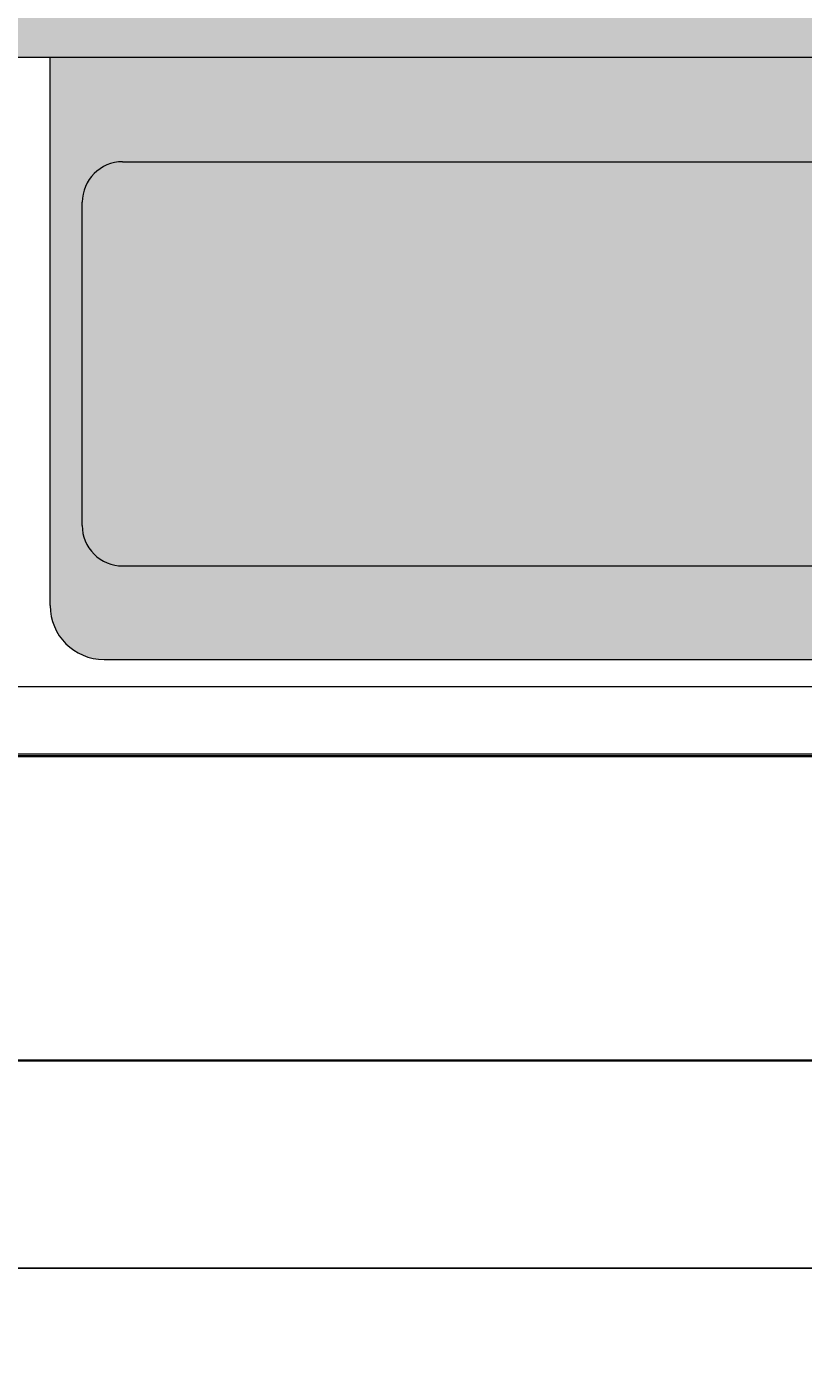
# Model space of a CAD drawing. Units: millimetres. Extents: x 27017497 to 27018854, y 7058029 to 7059154.
# Tile 21 of 91: x 27017679 to 27017702, y 7058124 to 7058163. Entities that reach past the tile are written whole.
import ezdxf

# ---------------------------------------------------------------- set-up
doc = ezdxf.new("R2010")
doc.units = ezdxf.units.MM
for name, color, linetype, lineweight in [('A-ANNO-DIMS', 2, 'Continuous', 18), ('A-FURN', 8, 'Continuous', 18), ('A-WALL', 7, 'Continuous', 35)]:
    doc.layers.add(name, color=color, linetype=linetype, lineweight=lineweight)
doc.layers.add('A-FURN-PATT', color=177, linetype='Continuous', lineweight=13, true_color=0x293189)
doc.styles.get("Standard").update_dxf_attribs({"font": 'arial.ttf'})
doc.dimstyles.get("Standard").update_dxf_attribs({"dimtxt": 0.18, "dimasz": 0.18, "dimexe": 0.18, "dimexo": 0.0625, "dimgap": 0.09, "dimtad": 0, "dimtih": 1, "dimtoh": 1, "dimdec": 4, "dimzin": 0, "dimdsep": 46, "dimtxsty": 'Standard', "dimcen": 0.09, "dimadec": 0, "dimazin": 0, "dimtfac": 1, "dimtdec": 4, "dimtofl": 0, "dimtmove": 0, "dimatfit": 3, "dimfxl": 1, "dimtolj": 1, "dimtzin": 0, "dimarcsym": 0})

# ---------------------------------------------------------------- blocks, each defined once
blk = doc.blocks.new('CAMMAT')
for p, q in [((1.27313, 0), (-1.27313, 0)), ((1.27313, -0.05), (-1.27313, -0.05)), ((0.61, -0.07), (-0.61, -0.07)), ((0.65, -0.11), (0.65, -0.51693)), ((0.59619, -0.1395), (0.05741, -0.1395)), ((0.62619, -0.1695), (0.62619, -0.4095)), ((0.59619, -0.4395), (0.05741, -0.4395)), ((-0.6904, -0.51693), (0.68256, -0.51693))]:
    blk.add_line(p, q)
for centre, radius, start, end in [((0.61, -0.11), 0.04, 0, 90), ((0.59619, -0.1695), 0.03, 360, 90), ((0.59619, -0.4095), 0.03, 270, 360)]:
    blk.add_arc(centre, radius, start, end)
blk = doc.blocks.new('*D25')
at = {"layer": 'A-ANNO-DIMS', "color": 0, "lineweight": -2, "transparency": 16777216}
for p, q in [((27017654.932, 7058141.917), (27017654.932, 7058126.587)), ((27017756.349, 7058141.917), (27017756.349, 7058126.587)), ((27017655.112, 7058126.767), (27017704.753, 7058126.767)), ((27017756.169, 7058126.767), (27017706.528, 7058126.767))]:
    blk.add_line(p, q, dxfattribs=at)
at = {"layer": 'A-ANNO-DIMS', "color": 0, "transparency": 16777216}
for points in [[(27017655.112, 7058126.797), (27017655.112, 7058126.737), (27017654.932, 7058126.767)], [(27017756.169, 7058126.797), (27017756.169, 7058126.737), (27017756.349, 7058126.767)]]:
    blk.add_solid(points, dxfattribs=at)
at = {"layer": 'Defpoints', "color": 0, "transparency": 16777216}
for p in [(27017654.932, 7058141.98), (27017756.349, 7058141.98), (27017654.932, 7058126.767)]:
    blk.add_point(p, dxfattribs=at)
at = {"layer": 'A-ANNO-DIMS', "color": 0, "transparency": 16777216, "insert": (27017705.64, 7058126.767), "char_height": 0.18, "attachment_point": 5}
blk.add_mtext('\\A1;BED 101 TYP.', dxfattribs=at)
blk = doc.blocks.new('*D47')
at = {"layer": 'A-ANNO-DIMS', "color": 0, "lineweight": -2, "transparency": 16777216}
for p, q in [((27017561.166, 7058294.35), (27017561.166, 7058028.6)), ((27018790.606, 7058294.35), (27018790.606, 7058028.6)), ((27017561.346, 7058028.78), (27018175.431, 7058028.78)), ((27018790.426, 7058028.78), (27018176.341, 7058028.78))]:
    blk.add_line(p, q, dxfattribs=at)
at = {"layer": 'A-ANNO-DIMS', "color": 0, "transparency": 16777216}
for points in [[(27017561.346, 7058028.81), (27017561.346, 7058028.75), (27017561.166, 7058028.78)], [(27018790.426, 7058028.81), (27018790.426, 7058028.75), (27018790.606, 7058028.78)]]:
    blk.add_solid(points, dxfattribs=at)
at = {"layer": 'Defpoints', "color": 0, "transparency": 16777216}
for p in [(27017561.166, 7058294.412), (27018790.606, 7058294.412), (27018790.606, 7058028.78)]:
    blk.add_point(p, dxfattribs=at)
at = {"layer": 'A-ANNO-DIMS', "color": 0, "transparency": 16777216, "insert": (27018175.886, 7058028.78), "char_height": 0.18, "attachment_point": 5}
blk.add_mtext('\\A1;1229.4', dxfattribs=at)
blk = doc.blocks.new('*D48')
at = {"layer": 'A-ANNO-DIMS', "color": 0, "lineweight": -2, "transparency": 16777216}
for p, q in [((27018463.498, 7058622.912), (27017497.536, 7058622.912)), ((27017497.716, 7058622.732), (27017497.716, 7058357.753)), ((27017497.716, 7058092.41), (27017497.716, 7058357.389)), ((27018555.129, 7058092.23), (27017497.536, 7058092.23))]:
    blk.add_line(p, q, dxfattribs=at)
at = {"layer": 'A-ANNO-DIMS', "color": 0, "transparency": 16777216}
for points in [[(27017497.686, 7058622.732), (27017497.746, 7058622.732), (27017497.716, 7058622.912)], [(27017497.686, 7058092.41), (27017497.746, 7058092.41), (27017497.716, 7058092.23)]]:
    blk.add_solid(points, dxfattribs=at)
at = {"layer": 'Defpoints', "color": 0, "transparency": 16777216}
for p in [(27018463.561, 7058622.912), (27017497.716, 7058092.23), (27018555.192, 7058092.23)]:
    blk.add_point(p, dxfattribs=at)
at = {"layer": 'A-ANNO-DIMS', "color": 0, "transparency": 16777216, "insert": (27017497.716, 7058357.571), "char_height": 0.18, "attachment_point": 5}
blk.add_mtext('\\A1;530.7', dxfattribs=at)

msp = doc.modelspace()

# ---------------------------------------------------------------- hatches: boundary and pattern name
at = {"layer": 'A-FURN-PATT'}
h = msp.add_hatch(color=256, dxfattribs=at)
h.dxf.hatch_style = 1
h.paths.add_polyline_path([(27017731.53, 7058218.852, 0.414214), (27017729.937, 7058220.445), (27017681.344, 7058220.445, 0.414214), (27017679.751, 7058218.852), (27017679.751, 7058174.658), (27017683.647, 7058174.959), (27017687.23, 7058175.46), (27017689.748, 7058176.196), (27017691.461, 7058177.277), (27017692.628, 7058178.816), (27017693.508, 7058180.922), (27017694.36, 7058183.707), (27017694.963, 7058180.902), (27017695.506, 7058178.662), (27017696.096, 7058176.759), (27017696.84, 7058174.966), (27017697.847, 7058173.059), (27017699.222, 7058170.809), (27017701.073, 7058167.99), (27017703.508, 7058164.376), (27017705.943, 7058167.99), (27017707.794, 7058170.809), (27017709.169, 7058173.059), (27017710.176, 7058174.966), (27017710.92, 7058176.759), (27017711.51, 7058178.662), (27017712.053, 7058180.902), (27017712.656, 7058183.707), (27017713.508, 7058180.922), (27017714.388, 7058178.816), (27017715.555, 7058177.277), (27017717.268, 7058176.196), (27017719.786, 7058175.46), (27017723.369, 7058174.959), (27017728.274, 7058174.58), (27017731.53, 7058174.396)])
h.paths.add_polyline_path([(27017723.369, 7058174.959), (27017719.786, 7058175.46), (27017717.268, 7058176.196), (27017715.555, 7058177.277), (27017714.388, 7058178.816), (27017713.508, 7058180.922), (27017712.656, 7058183.707), (27017712.053, 7058180.902), (27017711.51, 7058178.662), (27017710.92, 7058176.759), (27017710.176, 7058174.966), (27017709.169, 7058173.059), (27017707.794, 7058170.809), (27017705.943, 7058167.99), (27017703.508, 7058164.376), (27017734.763, 7058174.214), (27017728.274, 7058174.58)])
h.paths.add_polyline_path([(27017696.84, 7058174.966), (27017696.096, 7058176.759), (27017695.506, 7058178.662), (27017694.963, 7058180.902), (27017694.36, 7058183.707), (27017693.508, 7058180.922), (27017692.628, 7058178.816), (27017691.461, 7058177.277), (27017689.748, 7058176.196), (27017687.23, 7058175.46), (27017683.647, 7058174.959), (27017679.751, 7058174.658), (27017678.741, 7058174.58), (27017672.253, 7058174.214), (27017703.508, 7058164.376), (27017701.073, 7058167.99), (27017699.222, 7058170.809), (27017697.847, 7058173.059)])
h.paths.add_polyline_path([(27017678.454, 7058172.262), (27017678.454, 7058162.569), (27017733.139, 7058162.569), (27017733.139, 7058173.703), (27017703.508, 7058164.376)])
h.paths.add_polyline_path([(27017730.145, 7058158.291, 0.41419), (27017728.95, 7058159.485), (27017707.491, 7058159.485, 0.414214), (27017706.296, 7058158.29), (27017706.296, 7058148.731, 0.414214), (27017707.491, 7058147.536), (27017728.95, 7058147.536, 0.414237), (27017730.145, 7058148.731)], flags=0)
h.paths.add_polyline_path([(27017731.53, 7058162.569), (27017679.751, 7058162.569), (27017679.751, 7058146.361, 0.414214), (27017681.344, 7058144.768), (27017729.937, 7058144.768, 0.414214), (27017731.53, 7058146.361)])
h.paths.add_polyline_path([(27017703.354, 7058159.485, -0.41419), (27017704.549, 7058158.291), (27017704.549, 7058148.731, -0.414237), (27017703.354, 7058147.536), (27017681.894, 7058147.536, -0.41419), (27017680.699, 7058148.731), (27017680.699, 7058158.29, -0.414237), (27017681.894, 7058159.485)], flags=0)
h.paths.add_polyline_path([(27017707.491, 7058159.485), (27017728.95, 7058159.485, -0.41419), (27017730.145, 7058158.291), (27017730.145, 7058148.731, -0.414237), (27017728.95, 7058147.536), (27017707.491, 7058147.536, -0.414214), (27017706.296, 7058148.731), (27017706.296, 7058158.29, -0.414214)], flags=16)
h.paths.add_polyline_path([(27017704.549, 7058158.291, 0.41419), (27017703.354, 7058159.485), (27017681.894, 7058159.485, 0.414237), (27017680.699, 7058158.29), (27017680.699, 7058148.731, 0.41419), (27017681.894, 7058147.536), (27017703.354, 7058147.536, 0.414237), (27017704.549, 7058148.731)], flags=16)
h.paths.add_polyline_path([(27017752.64, 7058160.7), (27017732.725, 7058160.7), (27017732.725, 7058144.768), (27017752.64, 7058144.768)])
h.paths.add_polyline_path([(27017748.698, 7058152.101, -1), (27017736.749, 7058152.101, -1)], flags=16)
h.paths.add_polyline_path([(27017746.424, 7058152.101, -1), (27017739.024, 7058152.101, -1)], flags=0)
h.paths.add_polyline_path([(27017678.556, 7058160.7), (27017658.641, 7058160.7), (27017658.641, 7058144.768), (27017678.556, 7058144.768)])
h.paths.add_polyline_path([(27017674.806, 7058152.101, -1), (27017662.857, 7058152.101, -1)], flags=16)
h.paths.add_polyline_path([(27017672.531, 7058152.101, -1), (27017665.131, 7058152.101, -1)], flags=0)
h = msp.add_hatch(color=256, dxfattribs=at)
h.dxf.hatch_style = 1
h.paths.add_polyline_path([(27017730.145, 7058158.291, 0.41419), (27017728.95, 7058159.485), (27017707.491, 7058159.485, 0.414214), (27017706.296, 7058158.29), (27017706.296, 7058148.731, 0.414214), (27017707.491, 7058147.536), (27017728.95, 7058147.536, 0.414237), (27017730.145, 7058148.731)])
h.paths.add_polyline_path([(27017704.549, 7058158.291, 0.41419), (27017703.354, 7058159.485), (27017681.894, 7058159.485, 0.414237), (27017680.699, 7058158.29), (27017680.699, 7058148.731, 0.41419), (27017681.894, 7058147.536), (27017703.354, 7058147.536, 0.414237), (27017704.549, 7058148.731)])

# ---------------------------------------------------------------- linework, layer by layer
at = {"layer": 'A-WALL'}
for p, q in [((27017622.666, 7058141.912), (27017802.166, 7058141.912)), ((27017613.666, 7058132.912), (27017802.166, 7058132.912)), ((27017613.666, 7058132.912), (27017802.166, 7058132.912))]:
    msp.add_line(p, q, dxfattribs=at)

# ---------------------------------------------------------------- block references
at = {"layer": 'A-FURN', "xscale": 39.82996475819422, "yscale": 39.82996475819422, "zscale": 39.82996475819422, "rotation": 180}
msp.add_blockref('CAMMAT', (27017705.64, 7058141.98), dxfattribs=at)

# ---------------------------------------------------------------- dimensions: what is measured, and where the dimension line sits
at = {"layer": 'A-ANNO-DIMS'}
dim = msp.add_linear_dim(base=(27017497.716, 7058092.23), p1=(27018463.561, 7058622.912), p2=(27018555.192, 7058092.23), angle=90, dimstyle='Standard', override={"dimdec": 1, "dimlfac": 1, "dimrnd": 0, "dimzin": 0, "dimdsep": 46, "dimlunit": 2}, dxfattribs=at)
dim.commit()
dim.dimension.update_dxf_attribs({"geometry": '*D48', "text_midpoint": (27017497.716, 7058357.571)})
dim = msp.add_linear_dim(base=(27018790.606, 7058028.78), p1=(27017561.166, 7058294.412), p2=(27018790.606, 7058294.412), dimstyle='Standard', override={"dimdec": 1, "dimlfac": 1, "dimrnd": 0, "dimzin": 0, "dimdsep": 46, "dimlunit": 2}, dxfattribs=at)
dim.commit()
dim.dimension.update_dxf_attribs({"geometry": '*D47', "text_midpoint": (27018175.886, 7058028.78)})
dim = msp.add_linear_dim(base=(27017654.932, 7058126.767), p1=(27017756.349, 7058141.98), p2=(27017654.932, 7058141.98), angle=180, text='BED <> TYP.', dimstyle='Standard', override={"dimdec": 0, "dimlfac": 1, "dimrnd": 0, "dimzin": 0, "dimdsep": 46, "dimlunit": 2}, dxfattribs=at)
dim.commit()
dim.dimension.update_dxf_attribs({"geometry": '*D25', "text_midpoint": (27017705.64, 7058126.767)})

doc.saveas('drawing.dxf')
